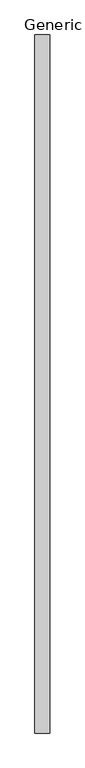
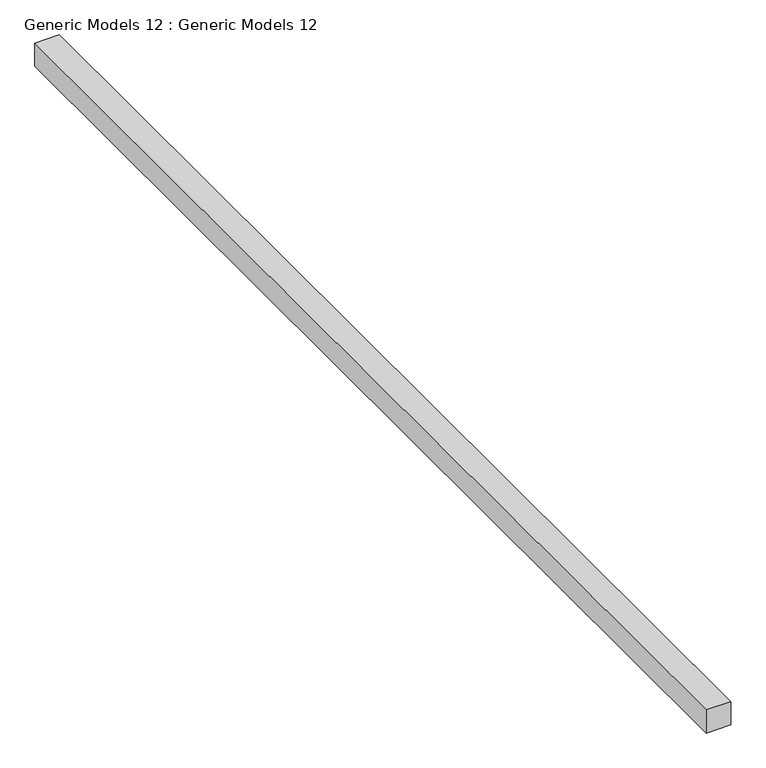
"""IFC4 building model written with IfcOpenShell, lengths in millimetres: proxy geometry, Generic Models 12 : Generic Models 12."""

from ifc_helpers import new_model, si_unit, frame, origin, place, context, project, spatial, polyline, outline, extrude, source, transform, mapped, element, save


def generic_models_12_generic_models_12_d8093b74(model_context):
    return source(origin(), model_context, "Body", "SweptSolid", [
        extrude(outline(polyline([(-14138.2638778, 2948.7988037), (-14138.2638778, 17410.2237525), (-13833.4638778, 17410.2237525), (-13833.4638778, 2948.7988037), (-14138.2638778, 2948.7988037)])), frame((0.0, 0.0, 6096.0), z_axis=(0.0, 0.0, 1.0), x_axis=(1.0, 0.0, 0.0)), (0.0, 0.0, 1.0), 304.8),
    ])


if __name__ == "__main__":
    model = new_model("IFC4")
    model_context = context("Model", 3, world=origin())
    ifc_project = project(units=[si_unit("LENGTHUNIT", "METRE", prefix="MILLI")], contexts=[model_context])
    site = spatial("IfcSite", under=ifc_project)
    building = spatial("IfcBuilding", under=site)
    placement = place(None, origin())
    generic_models_12_generic_models_12_shape = generic_models_12_generic_models_12_d8093b74(model_context)
    element("IfcBuildingElementProxy", 1, Name="Generic Models 12 : Generic Models 12", ObjectType="Generic Models 12 : Generic Models 12", at=placement, inside=building, context=model_context, shape_type="MappedRepresentation", body=[
        mapped(generic_models_12_generic_models_12_shape, transform((0.0, 0.0, 0.0), x_axis=(1.0, 0.0, 0.0), y_axis=(0.0, 1.0, 0.0), z_axis=(0.0, 0.0, 1.0))),
    ])
    save(model, "model.ifc")
